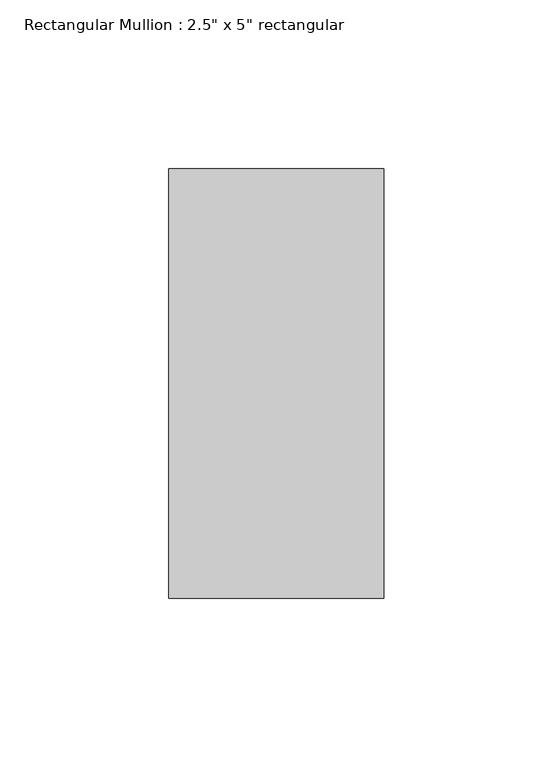
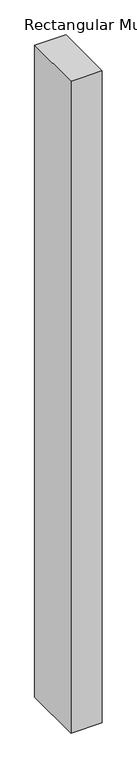
"""IFC4 building model written with IfcOpenShell, lengths in millimetres: member geometry."""

from ifc_helpers import new_model, si_unit, frame, origin, place, context, project, spatial, polyline, outline, extrude, source, transform, mapped, element, save


def member_f07b7441(model_context):
    return source(origin(), model_context, "Body", "SweptSolid", [
        extrude(outline(polyline([(0.0, 63.5), (0.0, -63.5), (-63.5, -63.5), (-63.5, 63.5), (0.0, 63.5)])), frame((0.0, 0.0, -1397.0), z_axis=(0.0, 0.0, 1.0), x_axis=(1.0, 0.0, 0.0)), (0.0, 0.0, 1.0), 1397.0),
    ])


if __name__ == "__main__":
    model = new_model("IFC4")
    model_context = context("Model", 3, world=origin())
    ifc_project = project(units=[si_unit("LENGTHUNIT", "METRE", prefix="MILLI")], contexts=[model_context])
    site = spatial("IfcSite", under=ifc_project)
    building = spatial("IfcBuilding", under=site)
    placement = place(None, origin())
    member_shape = member_f07b7441(model_context)
    element("IfcMember", 1, ObjectType="Rectangular Mullion : 2.5\" x 5\" rectangular", at=placement, inside=building, context=model_context, shape_type="MappedRepresentation", body=[
        mapped(member_shape, transform((0.0, 0.0, 0.0), x_axis=(1.0, 0.0, 0.0), y_axis=(0.0, 1.0, 0.0), z_axis=(0.0, 0.0, 1.0))),
    ])
    save(model, "model.ifc")

# Revit data of these elements
# Type "Rectangular Mullion : 2.5\" x 5\" rectangular"
#   built-in parameter 1007304 = 0.416667 (stored number, unit not read)
#   built-in parameter 1007301 = 0.104167 (stored number, unit not read)
#   built-in parameter 1007300 = 0.104167 (stored number, unit not read)
